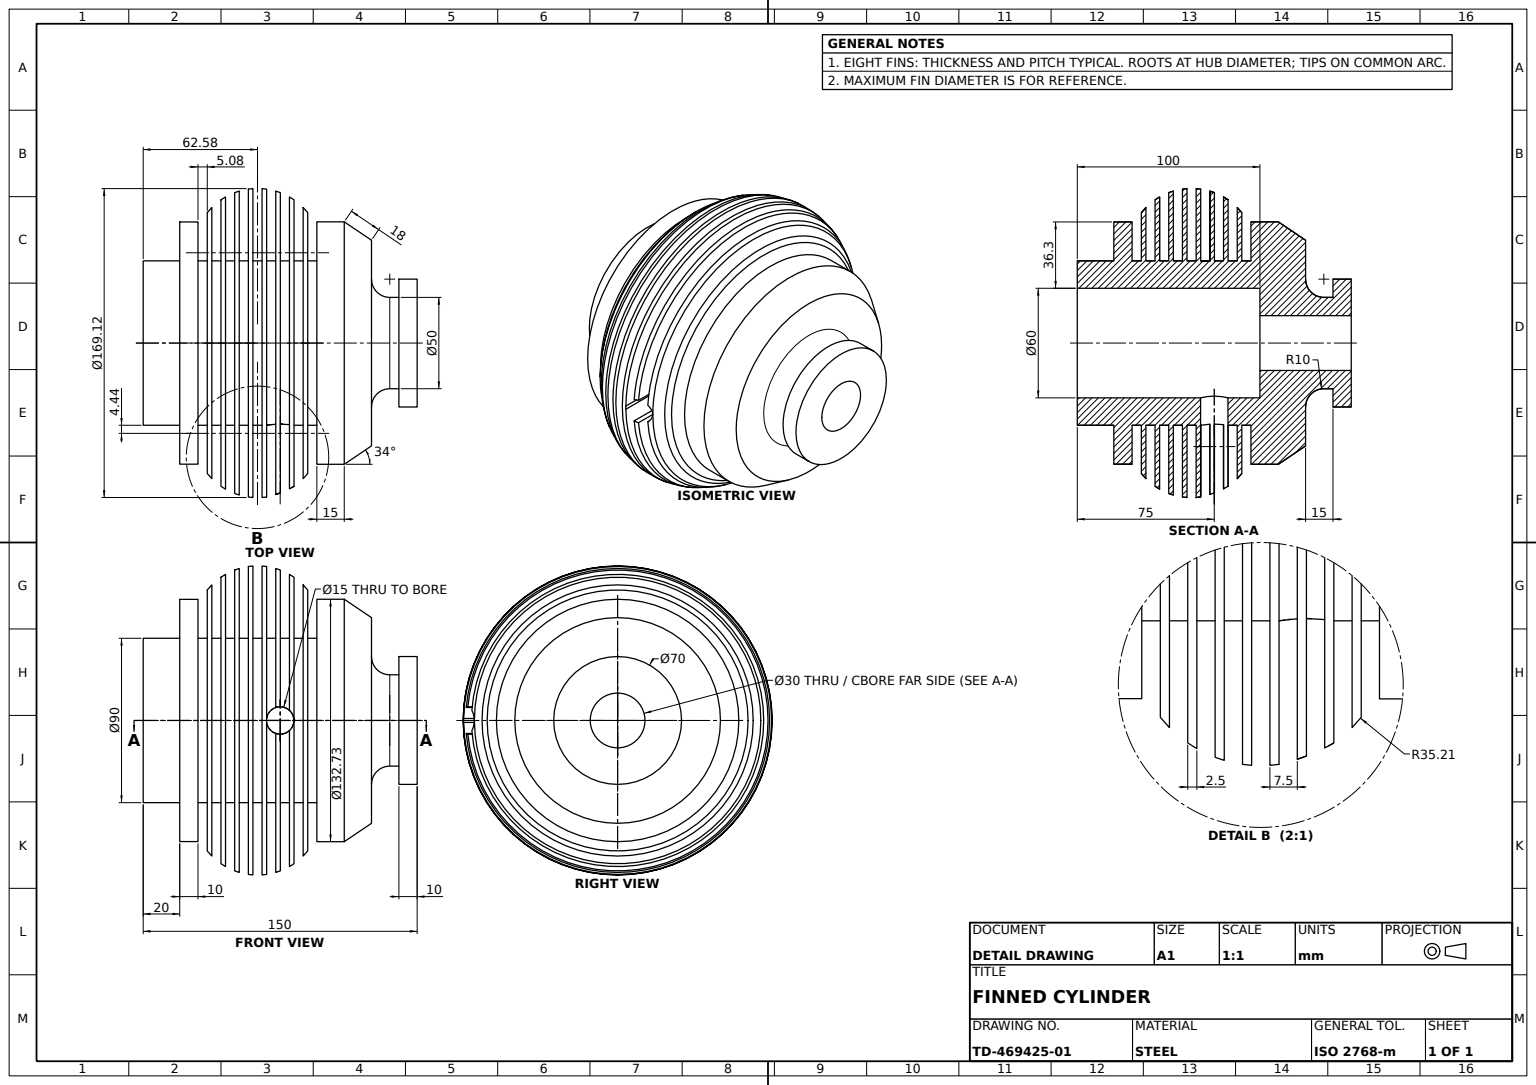
from build123d import *

# Parameters (mm, degrees)
THROUGH_BORE_PROFILE_R = 7.5
THROUGH_BORE_DEPTH     = 113


with BuildPart() as part:
    # Finned Body Profile → Finned Body Revolve (revolve)
    with BuildSketch(Plane.XY, mode=Mode.PRIVATE) as finned_body_revolve_sk:
        with BuildLine():
            Line((-2.343068637, 3.136106772), (-2.343068637, 23.136106772))
            Line((-2.343068637, 23.136106772), (7.656931363, 23.136106772))
            Line((7.656931363, 23.136106772), (7.656931363, 13.136106772))
            Line((7.656931363, 13.136106772), (12.656931363, 13.136106772))
            ThreePointArc((12.656931363, 13.136106772), (19.727999175, 16.06503896), (22.656931363, 23.136106772))
            Line((22.656931363, 23.136106772), (22.656931363, 44.436106772))
            Line((22.656931363, 44.436106772), (37.579607669, 54.501579034))
            Line((37.579607669, 54.501579034), (52.579607669, 54.501579034))
            Line((52.579607669, 54.501579034), (52.579607669, 33.136106772))
            Line((52.579607669, 33.136106772), (57.579607669, 33.136106772))
            Line((57.579607669, 33.136106772), (57.579607669, 59.559684826))
            ThreePointArc((57.579607669, 59.559684826), (58.792138591, 60.9961101), (60.079607669, 62.365771438))
            Line((60.079607669, 62.365771438), (60.079607669, 33.136106772))
            Line((60.079607669, 33.136106772), (65.079607669, 33.136106772))
            Line((65.079607669, 33.136106772), (65.079607669, 66.550701361))
            ThreePointArc((65.079607669, 66.550701361), (66.313077705, 67.364433648), (67.579607669, 68.125689463))
            Line((67.579607669, 68.125689463), (67.579607669, 33.136106772))
            Line((67.579607669, 33.136106772), (72.579607669, 33.136106772))
            Line((72.579607669, 33.136106772), (72.579607669, 70.489277526))
            ThreePointArc((72.579607669, 70.489277526), (73.821701113, 70.934558663), (75.079607669, 71.332983701))
            Line((75.079607669, 71.332983701), (75.079607669, 33.136106772))
            Line((75.079607669, 33.136106772), (80.079607669, 33.136106772))
            Line((80.079607669, 33.136106772), (80.079607669, 72.426166319))
            ThreePointArc((80.079607669, 72.426166319), (81.327214675, 72.582480256), (82.579607669, 72.694145278))
            Line((82.579607669, 72.694145278), (82.579607669, 33.136106772))
            Line((82.579607669, 33.136106772), (87.579607669, 33.136106772))
            Line((87.579607669, 33.136106772), (87.579607669, 72.694145278))
            ThreePointArc((87.579607669, 72.694145278), (88.832000663, 72.582480256), (90.079607669, 72.426166319))
            Line((90.079607669, 72.426166319), (90.079607669, 33.136106772))
            Line((90.079607669, 33.136106772), (95.079607669, 33.136106772))
            Line((95.079607669, 33.136106772), (95.079607669, 71.332983701))
            ThreePointArc((95.079607669, 71.332983701), (96.337514225, 70.934558663), (97.579607669, 70.489277526))
            Line((97.579607669, 70.489277526), (97.579607669, 33.136106772))
            Line((97.579607669, 33.136106772), (102.579607669, 33.136106772))
            Line((102.579607669, 33.136106772), (102.579607669, 68.125689463))
            ThreePointArc((102.579607669, 68.125689463), (103.846137633, 67.364433648), (105.079607669, 66.550701361))
            Line((105.079607669, 66.550701361), (105.079607669, 33.136106772))
            Line((105.079607669, 33.136106772), (110.079607669, 33.136106772))
            Line((110.079607669, 33.136106772), (110.079607669, 62.365771438))
            ThreePointArc((110.079607669, 62.365771438), (111.367076747, 60.9961101), (112.579607669, 59.559684826))
            Line((112.579607669, 59.559684826), (112.579607669, 33.136106772))
            Line((112.579607669, 33.136106772), (117.656931363, 33.136106772))
            Line((117.656931363, 33.136106772), (117.656931363, 54.436106772))
            Line((117.656931363, 54.436106772), (127.656931363, 54.436106772))
            Line((127.656931363, 54.436106772), (127.656931363, 33.136106772))
            Line((127.656931363, 33.136106772), (147.656931363, 33.136106772))
            Line((147.656931363, 33.136106772), (147.656931363, 18.136106772))
            Line((147.656931363, 18.136106772), (47.656931363, 18.136106772))
            Line((47.656931363, 18.136106772), (47.656931363, 3.136106772))
            Line((47.656931363, 3.136106772), (-2.343068637, 3.136106772))
        make_face()
    revolve(finned_body_revolve_sk.sketch.rotate(Axis((-190.290293796, -11.863893228, 0), (1, 0, 0)), 90), axis=Axis((-190.290293796, -11.863893228, 0), (1, 0, 0)))

    # Through Bore Profile → Through Bore (cut)
    with BuildSketch(Plane.XY):
        with Locations((72.656931363, -11.863893228)):
            Circle(THROUGH_BORE_PROFILE_R)
    extrude(amount=-THROUGH_BORE_DEPTH, mode=Mode.SUBTRACT)


solid = part.part
